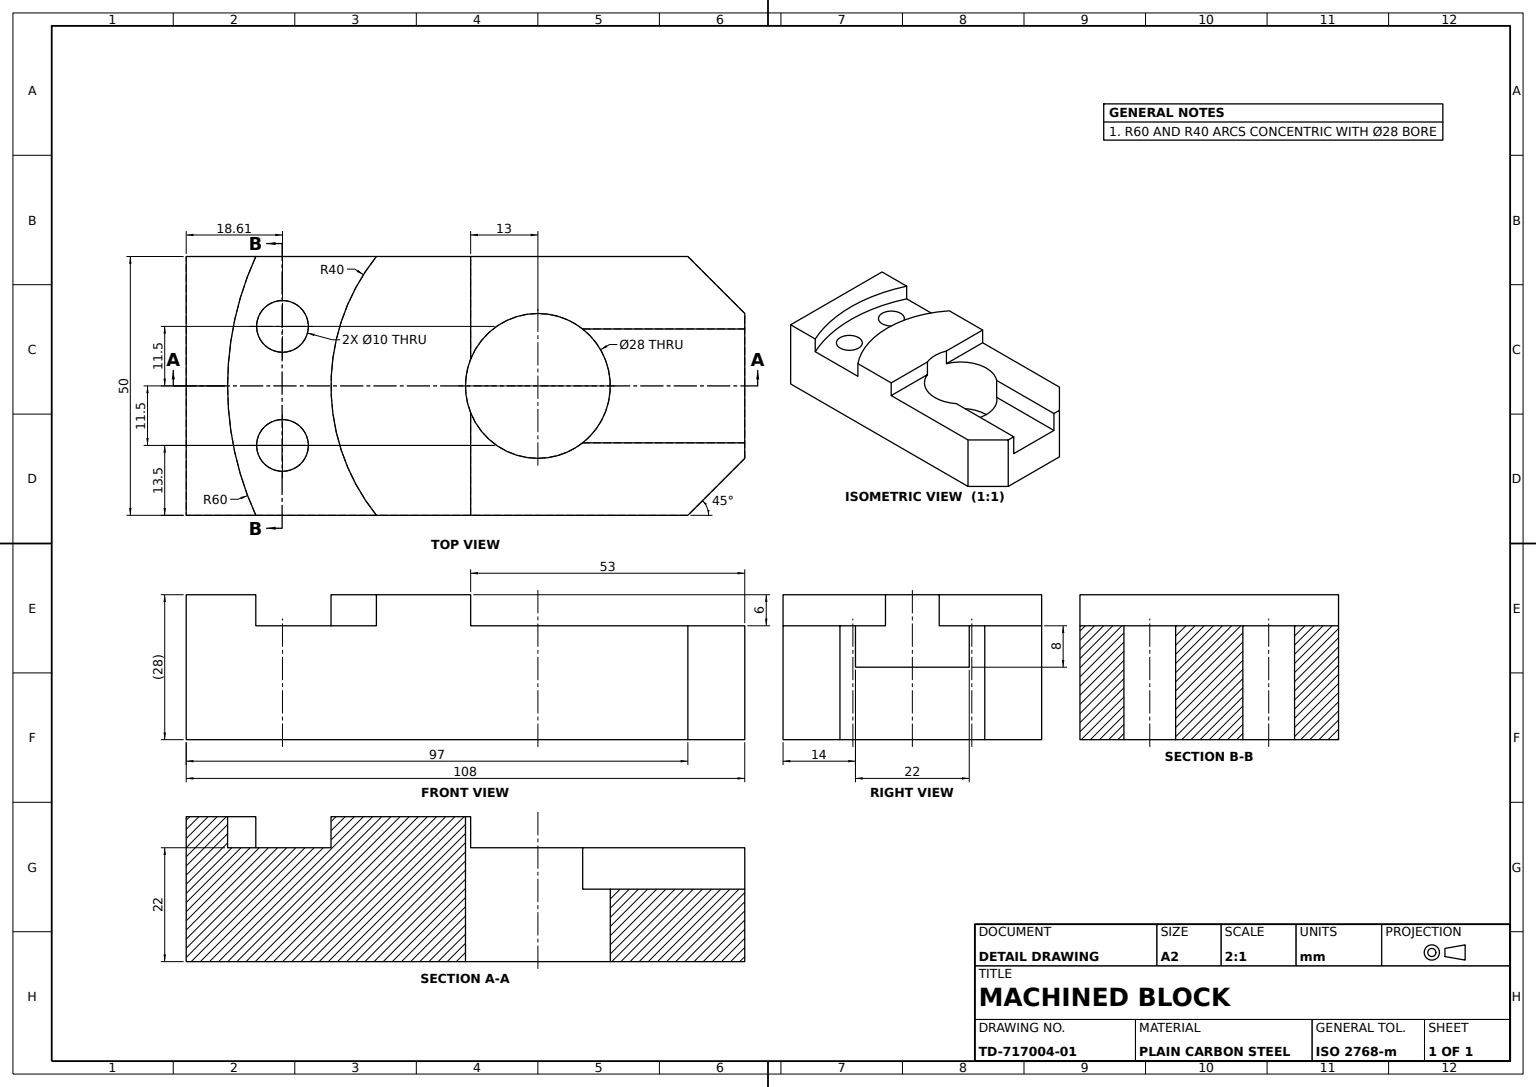
from build123d import *

# Parameters (mm, degrees)
BASE_BLOCK_108X50X28_DEPTH     = 28
JAW_SLOT_PROFILE_W             = 22
JAW_SLOT_PROFILE_H             = 6
JAW_SLOT_CUT_DEPTH             = 40
BORE_28_PROFILE_R              = 14
BORE_28_DEPTH                  = 66.76473219
THROUGH_SLOT_CUT_DEPTH         = 53
SIDE_GROOVE_PROFILE_W          = 22
SIDE_GROOVE_PROFILE_H          = 8
SIDE_GROOVE_CUT_DEPTH          = 40
END_CHAMFER_11X45_SIZE         = 11
ARC_RECESS_6_DEEP_DEPTH        = 6
ARC_POCKET_AND_HOLES_PROFILE_R = 5
ARC_POCKET_AND_HOLES_CUT_DEPTH = 66.76473219


with BuildPart() as part:
    # Base Block Profile → Base Block 108x50x28 (new body)
    with BuildSketch(Plane(origin=(0, 0, 0), x_dir=(1, 0, 0), z_dir=(0, 1, 0))):
        Polygon((-54, 25), (43, 25), (54, 25), (54, -25), (43, -25), (-54, -25), align=None)
    extrude(amount=BASE_BLOCK_108X50X28_DEPTH)

    # Jaw Slot Profile → Jaw Slot Cut (cut)
    with BuildSketch(Plane(origin=(54, 0, 0), x_dir=(0, 0, -1), z_dir=(1, 0, 0))):
        with Locations((0, 25)):
            Rectangle(JAW_SLOT_PROFILE_W, JAW_SLOT_PROFILE_H)
    extrude(amount=-JAW_SLOT_CUT_DEPTH, mode=Mode.SUBTRACT)

    # Bore Ø28 Profile → Bore Ø28 (cut, through all)
    with BuildSketch(Plane(origin=(0, 28, 0), x_dir=(1, 0, 0), z_dir=(0, 1, 0))):
        with Locations(Location((14, 0, 0), (0, 0, 270))):
            Circle(BORE_28_PROFILE_R)
    extrude(amount=-BORE_28_DEPTH, mode=Mode.SUBTRACT)

    # Through Slot Profile → Through Slot Cut (cut)
    with BuildSketch(Plane(origin=(54, 0, 0), x_dir=(0, 0, -1), z_dir=(1, 0, 0))):
        Polygon((-25, 28), (-11, 28), (25, 28), (25, 22), (-11, 22), (-25, 22), align=None)
    extrude(amount=-THROUGH_SLOT_CUT_DEPTH, mode=Mode.SUBTRACT)

    # Side Groove Profile → Side Groove Cut (cut)
    with BuildSketch(Plane(origin=(54, 0, 0), x_dir=(0, 0, -1), z_dir=(1, 0, 0))):
        with Locations((0, 18)):
            Rectangle(SIDE_GROOVE_PROFILE_W, SIDE_GROOVE_PROFILE_H)
    extrude(amount=-SIDE_GROOVE_CUT_DEPTH, mode=Mode.SUBTRACT)

    # End Chamfer 11x45°
    end_chamfer_11x45_edges = [part.edges().sort_by_distance(p)[0] for p in [
        (54, 11, 25),
        (54, 11, -25),
    ]]
    chamfer(end_chamfer_11x45_edges, length=END_CHAMFER_11X45_SIZE)

    # Arc Recess Profile → Arc Recess 6 Deep (cut)
    with BuildSketch(Plane(origin=(0, 28, 0), x_dir=(1, 0, 0), z_dir=(0, 1, 0))):
        with BuildLine():
            Line((-40.543560573, -25), (-17.224989992, -25))
            ThreePointArc((-17.224989992, -25), (-26, 0), (-17.224989992, 25))
            Line((-17.224989992, 25), (-40.543560573, 25))
            ThreePointArc((-40.543560573, 25), (-46, 0), (-40.543560573, -25))
        make_face()
    extrude(amount=-ARC_RECESS_6_DEEP_DEPTH, mode=Mode.SUBTRACT)

    # Arc Pocket and Holes Profile → Arc Pocket and Holes Cut (cut, through all)
    with BuildSketch(Plane(origin=(0, 28, 0), x_dir=(1, 0, 0), z_dir=(0, 1, 0))):
        with Locations(Location((-35.385362758, 11.497401318, 0), (0, 0, 270))):
            Circle(ARC_POCKET_AND_HOLES_PROFILE_R)
        with Locations(Location((-35.385362758, -11.497401318, 0), (0, 0, 270))):
            Circle(ARC_POCKET_AND_HOLES_PROFILE_R)
    extrude(amount=-ARC_POCKET_AND_HOLES_CUT_DEPTH, mode=Mode.SUBTRACT)


solid = part.part
